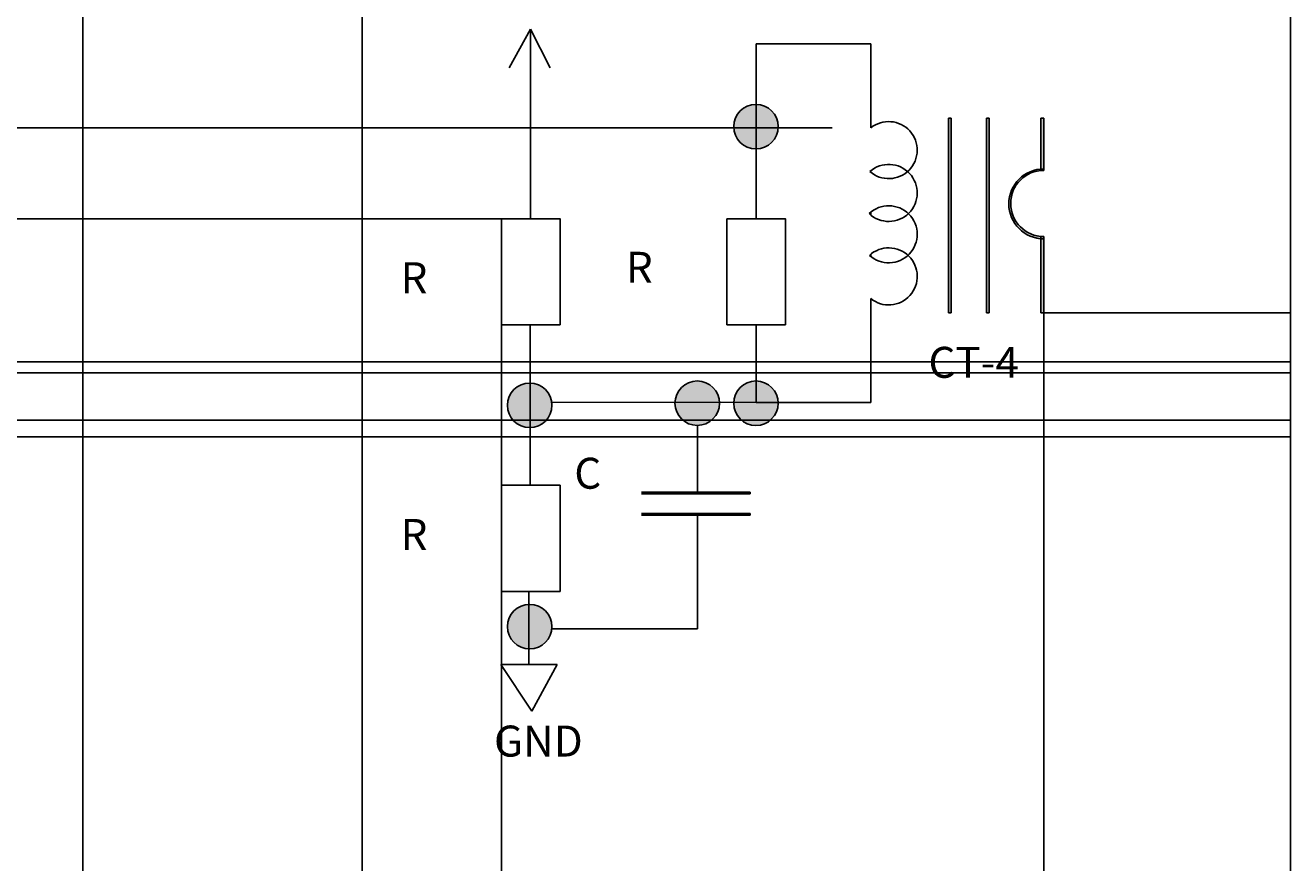
# Model space of a CAD drawing. Units: inches. Extents: x 35362 to 73946, y 43607 to 67532.
# Tile 133 of 134: x 64925 to 73946, y 49781 to 55752. Entities that reach past the tile are written whole.
import ezdxf

# ---------------------------------------------------------------- set-up
doc = ezdxf.new("R2010")
doc.units = ezdxf.units.IN
doc.header["$MEASUREMENT"] = 0
for name, color, linetype, lineweight in [('A-ANNO-DIMS', 2, 'Continuous', 18), ('E-ANNO-TEXT', 5, 'Continuous', 18), ('E-SYMB', 1, 'Continuous', 25), ('E-SYMB-PATT', 1, 'Continuous', 13), ('E-WIRE', 3, 'Continuous', 25)]:
    doc.layers.add(name, color=color, linetype=linetype, lineweight=lineweight)
doc.styles.get("Standard").update_dxf_attribs({"font": 'arial.ttf'})
doc.dimstyles.get("Standard").update_dxf_attribs({"dimtxt": 0.18, "dimasz": 0.18, "dimexe": 0.18, "dimexo": 0.0625, "dimgap": 0.09, "dimtad": 0, "dimtih": 1, "dimtoh": 1, "dimdec": 4, "dimzin": 0, "dimdsep": 46, "dimtxsty": 'Standard', "dimcen": 0.09, "dimadec": 0, "dimazin": 0, "dimtfac": 1, "dimtdec": 4, "dimtofl": 0, "dimtmove": 0, "dimatfit": 3, "dimfxl": 1, "dimtolj": 1, "dimtzin": 0, "dimarcsym": 0})

# ---------------------------------------------------------------- blocks, each defined once
blk = doc.blocks.new('CT-CORE')
for p, q in [((-0.0004610742907971, 1387.996120092102), (-0.0004610742907971, -5.34733626409e-05)), ((19.99953892572375, 1387.996120092102), (-0.0004610742907971, 1387.996120092102)), ((19.9995389257092, -5.34733626409e-05), (19.99953892572375, 1387.996120092102)), ((270.6681283192447, 1387.996120092102), (270.6681283192447, -5.34733626409e-05)), ((290.6681283192593, 1387.996120092102), (270.6681283192447, 1387.996120092102)), ((290.6681283192447, -5.34733626409e-05), (290.6681283192593, 1387.996120092102)), ((658.9826659540267, 1387.996120092102), (658.9826659540267, 1014.585417332389)), ((678.9826659540413, 1387.996120092102), (658.9826659540267, 1387.996120092102)), ((678.9826659540413, 1015.434583844784), (678.9826659540413, 1387.996120092102)), ((658.9826659540267, 544.3844491987692), (658.9826659540267, -5.34733626409e-05)), ((678.9826659540267, -5.34733626409e-05), (678.9826659540413, 543.5352826863744)), ((-0.0004610742907971, -5.34733626409e-05), (19.9995389257092, -5.34733626409e-05)), ((270.6681283192447, -5.34733626409e-05), (290.6681283192447, -5.34733626409e-05)), ((658.9826659540267, -5.34733626409e-05), (678.9826659540267, -5.34733626409e-05))]:
    blk.add_line(p, q)
blk.add_arc((678.9826659540267, 779.4849332655793), 235.9496505792049, 90, 270)
blk = doc.blocks.new('PWR-5V')
for p, q in [((149.83075954589, 1350.920325582869), (-0.0001436721213395, 1075.898385659784)), ((149.83075954589, 833.0941938853575), (149.83075954589, 1350.920325582869)), ((289.9554714129044, 1075.898385659784), (149.83075954589, 1350.920325582869)), ((149.83075954589, 416.3126341884199), (149.83075954589, 833.0941938853575)), ((149.83075954589, 416.3126341884199), (149.83075954589, 0.0003315384019515))]:
    blk.add_line(p, q)
blk = doc.blocks.new('*D6')
at = {"layer": 'A-ANNO-DIMS', "color": 0, "lineweight": -2, "transparency": 16777216}
for p, q in [((72185.645666, 53702.123839), (72185.645666, 43606.678996)), ((69871.496302, 45449.831951), (69871.496302, 43606.678996)), ((69871.67630199999, 43606.858996), (71028.21104539152, 43606.858996)), ((72185.465666, 43606.858996), (71028.93092260844, 43606.858996))]:
    blk.add_line(p, q, dxfattribs=at)
at = {"layer": 'A-ANNO-DIMS', "color": 0, "transparency": 16777216}
for points in [[(69871.67630199999, 43606.888996), (69871.67630199999, 43606.828996), (69871.496302, 43606.858996)], [(72185.465666, 43606.888996), (72185.465666, 43606.828996), (72185.645666, 43606.858996)]]:
    blk.add_solid(points, dxfattribs=at)
at = {"layer": 'Defpoints', "color": 0, "transparency": 16777216}
for p in [(72185.645666, 53702.186339), (69871.496302, 45449.894451), (72185.645666, 43606.858996)]:
    blk.add_point(p, dxfattribs=at)
at = {"layer": 'A-ANNO-DIMS', "color": 0, "transparency": 16777216, "insert": (71028.57098399999, 43606.858996), "char_height": 0.18, "attachment_point": 5}
blk.add_mtext('\\A1;2314', dxfattribs=at)
blk = doc.blocks.new('*D7')
at = {"layer": 'A-ANNO-DIMS', "color": 0, "lineweight": -2, "transparency": 16777216}
for p, q in [((72185.70816600003, 53702.18633900003), (73945.82566600003, 53702.18633900003)), ((73945.64566600005, 53702.00633900003), (73945.64566600005, 49576.22229813781)), ((73945.64566600005, 45450.07445100001), (73945.64566600005, 49575.85849186223)), ((69871.55880200003, 45449.89445100001), (73945.82566600003, 45449.89445100001))]:
    blk.add_line(p, q, dxfattribs=at)
at = {"layer": 'A-ANNO-DIMS', "color": 0, "transparency": 16777216}
for points in [[(73945.61566600006, 53702.00633900003), (73945.67566600005, 53702.00633900003), (73945.64566600005, 53702.18633900003)], [(73945.61566600006, 45450.07445100001), (73945.67566600005, 45450.07445100001), (73945.64566600005, 45449.89445100001)]]:
    blk.add_solid(points, dxfattribs=at)
at = {"layer": 'Defpoints', "color": 0, "transparency": 16777216}
for p in [(72185.64566600003, 53702.18633900003), (73945.64566600005, 53702.18633900003), (69871.49630200001, 45449.89445100001)]:
    blk.add_point(p, dxfattribs=at)
at = {"layer": 'A-ANNO-DIMS', "color": 0, "transparency": 16777216, "insert": (73945.64566600005, 49576.04039499998), "char_height": 0.18, "attachment_point": 5}
blk.add_mtext('\\A1;8252', dxfattribs=at)
blk = doc.blocks.new('*D8')
at = {"layer": 'A-ANNO-DIMS', "color": 0, "lineweight": -2, "transparency": 16777216}
for p, q in [((66271.28651900003, 65771.51172800003), (73945.82566600003, 65771.51172800003)), ((73945.64566600005, 65771.33172800003), (73945.64566600005, 59737.03093663782)), ((73945.64566600005, 53702.36633900002), (73945.64566600005, 59736.66713036224)), ((72185.70816600003, 53702.18633900003), (73945.82566600003, 53702.18633900003))]:
    blk.add_line(p, q, dxfattribs=at)
at = {"layer": 'A-ANNO-DIMS', "color": 0, "transparency": 16777216}
for points in [[(73945.61566600006, 65771.33172800003), (73945.67566600005, 65771.33172800003), (73945.64566600005, 65771.51172800003)], [(73945.61566600006, 53702.36633900002), (73945.67566600005, 53702.36633900002), (73945.64566600005, 53702.18633900003)]]:
    blk.add_solid(points, dxfattribs=at)
at = {"layer": 'Defpoints', "color": 0, "transparency": 16777216}
for p in [(66271.22401900003, 65771.51172800003), (73945.64566600005, 65771.51172800003), (72185.64566600003, 53702.18633900003)]:
    blk.add_point(p, dxfattribs=at)
at = {"layer": 'A-ANNO-DIMS', "color": 0, "transparency": 16777216, "insert": (73945.64566600005, 59736.84903349999), "char_height": 0.18, "attachment_point": 5}
blk.add_mtext('\\A1;12069', dxfattribs=at)
blk = doc.blocks.new('*D10')
at = {"layer": 'A-ANNO-DIMS', "color": 0, "lineweight": -2, "transparency": 16777216}
for p, q in [((61240.96983600002, 59185.14395700003), (73945.82566600003, 59185.14395700003)), ((73945.64566600005, 59184.96395700003), (73945.64566600005, 56268.51827402935)), ((73945.64566600005, 53351.70866200003), (73945.64566600005, 56268.1543449707)), ((61240.96983600002, 53351.52866200003), (73945.82566600003, 53351.52866200003))]:
    blk.add_line(p, q, dxfattribs=at)
at = {"layer": 'A-ANNO-DIMS', "color": 0, "transparency": 16777216}
for points in [[(73945.61566600006, 59184.96395700003), (73945.67566600005, 59184.96395700003), (73945.64566600005, 59185.14395700003)], [(73945.61566600006, 53351.70866200003), (73945.67566600005, 53351.70866200003), (73945.64566600005, 53351.52866200003)]]:
    blk.add_solid(points, dxfattribs=at)
at = {"layer": 'Defpoints', "color": 0, "transparency": 16777216}
for p in [(61240.90733600002, 59185.14395700003), (61240.90733600002, 53351.52866200003), (73945.64566600005, 53351.52866200003)]:
    blk.add_point(p, dxfattribs=at)
at = {"layer": 'A-ANNO-DIMS', "color": 0, "transparency": 16777216, "insert": (73945.64566600005, 56268.33630949999), "char_height": 0.18, "attachment_point": 5}
blk.add_mtext('\\A1;5834', dxfattribs=at)
blk = doc.blocks.new('*D36')
at = {"layer": 'A-ANNO-DIMS', "color": 0, "lineweight": -2, "transparency": 16777216}
for p, q in [((68320.80826200004, 60122.34633200002), (35361.76908500003, 60122.34633200002)), ((35361.94908500003, 60122.16633200002), (35361.94908500003, 57247.82893113781)), ((35361.94908500003, 54373.12772400002), (35361.94908500003, 57247.46512486223)), ((68320.80826200004, 54372.94772400003), (35361.76908500003, 54372.94772400002))]:
    blk.add_line(p, q, dxfattribs=at)
at = {"layer": 'A-ANNO-DIMS', "color": 0, "transparency": 16777216}
for points in [[(35361.91908500003, 60122.16633200002), (35361.97908500003, 60122.16633200002), (35361.94908500003, 60122.34633200002)], [(35361.91908500003, 54373.12772400002), (35361.97908500003, 54373.12772400002), (35361.94908500003, 54372.94772400002)]]:
    blk.add_solid(points, dxfattribs=at)
at = {"layer": 'Defpoints', "color": 0, "transparency": 16777216}
for p in [(68320.87076200004, 60122.34633200002), (35361.94908500003, 54372.94772400002), (68320.87076200004, 54372.94772400003)]:
    blk.add_point(p, dxfattribs=at)
at = {"layer": 'A-ANNO-DIMS', "color": 0, "transparency": 16777216, "insert": (35361.94908500004, 57247.64702799999), "char_height": 0.18, "attachment_point": 5}
blk.add_mtext('\\A1;5749.4', dxfattribs=at)
blk = doc.blocks.new('*D56')
at = {"layer": 'A-ANNO-DIMS', "color": 0, "lineweight": -2, "transparency": 16777216}
for p, q in [((59433.20767900003, 53351.52866200003), (73945.82566600003, 53351.52866200003)), ((73945.64566600005, 53351.34866200002), (73945.64566600005, 53143.55447552935)), ((73945.64566600005, 52935.39636000002), (73945.64566600005, 53143.19054647069)), ((59433.20767900003, 52935.21636000003), (73945.82566600003, 52935.21636000003))]:
    blk.add_line(p, q, dxfattribs=at)
at = {"layer": 'A-ANNO-DIMS', "color": 0, "transparency": 16777216}
for points in [[(73945.61566600006, 53351.34866200002), (73945.67566600005, 53351.34866200002), (73945.64566600005, 53351.52866200003)], [(73945.61566600006, 52935.39636000002), (73945.67566600005, 52935.39636000002), (73945.64566600005, 52935.21636000003)]]:
    blk.add_solid(points, dxfattribs=at)
at = {"layer": 'Defpoints', "color": 0, "transparency": 16777216}
for p in [(59433.14517900002, 53351.52866200003), (59433.14517900002, 52935.21636000003), (73945.64566600005, 52935.21636000003)]:
    blk.add_point(p, dxfattribs=at)
at = {"layer": 'A-ANNO-DIMS', "color": 0, "transparency": 16777216, "insert": (73945.64566600005, 53143.37251099998), "char_height": 0.18, "attachment_point": 5}
blk.add_mtext('\\A1;416.3', dxfattribs=at)
blk = doc.blocks.new('*D57')
at = {"layer": 'A-ANNO-DIMS', "color": 0, "lineweight": -2, "transparency": 16777216}
for p, q in [((51445.41811300003, 53272.78194700003), (73945.82566600003, 53272.78194700003)), ((73945.64566600005, 53272.60194700003), (73945.64566600005, 53045.85764863782)), ((73945.64566600005, 52818.74954400002), (73945.64566600005, 53045.49384236224)), ((51445.41811300003, 52818.56954400002), (73945.82566600003, 52818.56954400002))]:
    blk.add_line(p, q, dxfattribs=at)
at = {"layer": 'A-ANNO-DIMS', "color": 0, "transparency": 16777216}
for points in [[(73945.61566600006, 53272.60194700003), (73945.67566600005, 53272.60194700003), (73945.64566600005, 53272.78194700003)], [(73945.61566600006, 52818.74954400002), (73945.67566600005, 52818.74954400002), (73945.64566600005, 52818.56954400002)]]:
    blk.add_solid(points, dxfattribs=at)
at = {"layer": 'Defpoints', "color": 0, "transparency": 16777216}
for p in [(51445.35561300003, 53272.78194700003), (51445.35561300003, 52818.56954400002), (73945.64566600005, 52818.56954400002)]:
    blk.add_point(p, dxfattribs=at)
at = {"layer": 'A-ANNO-DIMS', "color": 0, "transparency": 16777216, "insert": (73945.64566600005, 53045.6757455), "char_height": 0.18, "attachment_point": 5}
blk.add_mtext('\\A1;454.2', dxfattribs=at)
blk = doc.blocks.new('*D65')
at = {"layer": 'A-ANNO-DIMS', "color": 0, "lineweight": -2, "transparency": 16777216}
for p, q in [((65336.01600799999, 61293.223552), (65336.01600799999, 43606.678996)), ((67326.639741, 61293.223552), (67326.639741, 43606.678996)), ((65336.19600799999, 43606.858996), (66330.87277900206, 43606.858996)), ((67326.45974100001, 43606.858996), (66331.78296999796, 43606.858996))]:
    blk.add_line(p, q, dxfattribs=at)
at = {"layer": 'A-ANNO-DIMS', "color": 0, "transparency": 16777216}
for points in [[(65336.19600799999, 43606.888996), (65336.19600799999, 43606.828996), (65336.01600799999, 43606.858996)], [(67326.45974100001, 43606.888996), (67326.45974100001, 43606.828996), (67326.639741, 43606.858996)]]:
    blk.add_solid(points, dxfattribs=at)
at = {"layer": 'Defpoints', "color": 0, "transparency": 16777216}
for p in [(65336.01600799999, 61293.286052), (67326.639741, 61293.286052), (67326.639741, 43606.858996)]:
    blk.add_point(p, dxfattribs=at)
at = {"layer": 'A-ANNO-DIMS', "color": 0, "transparency": 16777216, "insert": (66331.32787450001, 43606.858996), "char_height": 0.18, "attachment_point": 5}
blk.add_mtext('\\A1;1990.6', dxfattribs=at)
blk = doc.blocks.new('*D68')
at = {"layer": 'A-ANNO-DIMS', "color": 0, "lineweight": -2, "transparency": 16777216}
for p, q in [((68320.870762, 54372.885224), (68320.870762, 43606.678996)), ((61240.907336, 53351.466162), (61240.907336, 43606.678996)), ((61241.08733599999, 43606.858996), (64780.42646373397, 43606.858996)), ((68320.69076200001, 43606.858996), (64781.35163426603, 43606.858996))]:
    blk.add_line(p, q, dxfattribs=at)
at = {"layer": 'A-ANNO-DIMS', "color": 0, "transparency": 16777216}
for points in [[(61241.08733599999, 43606.888996), (61241.08733599999, 43606.828996), (61240.907336, 43606.858996)], [(68320.69076200001, 43606.888996), (68320.69076200001, 43606.828996), (68320.870762, 43606.858996)]]:
    blk.add_solid(points, dxfattribs=at)
at = {"layer": 'Defpoints', "color": 0, "transparency": 16777216}
for p in [(68320.870762, 54372.947724), (61240.907336, 53351.52866199999), (68320.870762, 43606.858996)]:
    blk.add_point(p, dxfattribs=at)
at = {"layer": 'A-ANNO-DIMS', "color": 0, "transparency": 16777216, "insert": (64780.889049, 43606.858996), "char_height": 0.18, "attachment_point": 5}
blk.add_mtext('\\A1;7080.0', dxfattribs=at)

msp = doc.modelspace()

# ---------------------------------------------------------------- hatches: boundary and pattern name
at = {"layer": 'E-SYMB-PATT'}
h = msp.add_hatch(color=256, dxfattribs=at)
h.dxf.hatch_style = 1
h.paths.add_polyline_path([(70135.80528894292, 55188.08141031771, 0.4183931940818975), (69974.93949760578, 55029.49162493918, 0.4183931940818975), (70135.80528894292, 54870.90183956064)])
h.paths.add_polyline_path([(70135.80528894292, 55188.08141031771), (70135.80528894292, 54870.90183956064, 0.4100462469397049), (70292.15127038094, 55029.49162493918, 0.4100462469397049)])
h = msp.add_hatch(color=256, dxfattribs=at)
h.dxf.hatch_style = 1
h.paths.add_polyline_path([(71526.66253892572, 55090.18251302161), (71506.66253892571, 55090.18251302161), (71506.66253892571, 53702.18633945615), (71526.6625389257, 53702.18633945615)])
h = msp.add_hatch(color=256, dxfattribs=at)
h.dxf.hatch_style = 1
h.paths.add_polyline_path([(71797.33112831926, 55090.18251302161), (71777.33112831925, 55090.18251302161), (71777.33112831925, 53702.18633945615), (71797.33112831925, 53702.18633945615)])
h = msp.add_hatch(color=256, dxfattribs=at)
h.dxf.hatch_style = 1
h.paths.add_polyline_path([(72185.64566595404, 54245.72167561588, -0.0212196039209565), (72165.64566595403, 54246.57084212828), (72165.64566595403, 54229.69792765927, 0.0200709024740955), (72185.64566595404, 54228.89476801458)])
h.paths.add_polyline_path([(72185.64566595404, 54228.89476801458, -0.0200709024740953), (72165.64566595403, 54229.69792765927), (72165.64566595403, 53702.18633945615), (72185.64566595403, 53702.18633945615)])
h.paths.add_polyline_path([(72185.64566595404, 55090.18251302161), (72165.64566595403, 55090.18251302161), (72165.64566595403, 54726.92775889016, -0.0200709024740959), (72185.64566595404, 54727.73091853485)])
h.paths.add_polyline_path([(72185.64566595404, 54727.73091853485, 0.020070902474096), (72165.64566595403, 54726.92775889015), (72165.64566595403, 54716.77181026191, -0.0212196039209564), (72185.64566595404, 54717.62097677429)])
h = msp.add_hatch(color=256, dxfattribs=at)
h.dxf.hatch_style = 1
h.paths.add_polyline_path([(72165.64566595403, 54716.77181026191), (72165.64566595403, 54726.92775889016, 0.3908929169039177), (71936.22759069389, 54478.31284327471, 0.3908929169039177), (72165.64566595403, 54229.69792765927), (72165.64566595403, 54246.57084212828, -0.389569854577291), (71949.69601537482, 54481.67132619509, -0.389569854577291)])
h = msp.add_hatch(color=256, dxfattribs=at)
h.dxf.hatch_style = 1
h.paths.add_polyline_path([(68522.99328781641, 53200.70415181951, 0.4183931940818975), (68362.12749647925, 53042.11436644098, 0.4183931940818975), (68522.99328781641, 52883.52458106244)])
h.paths.add_polyline_path([(68522.99328781641, 53200.70415181951), (68522.99328781641, 52883.52458106244, 0.4100462469397049), (68679.33926925441, 53042.11436644098, 0.4100462469397049)])
h = msp.add_hatch(color=256, dxfattribs=at)
h.dxf.hatch_style = 1
h.paths.add_polyline_path([(69717.45127656072, 53215.91996812531, 0.4183931940818975), (69556.58548522356, 53057.33018274678, 0.4183931940818975), (69717.45127656072, 52898.74039736824)])
h.paths.add_polyline_path([(69717.45127656072, 53215.91996812531), (69717.45127656072, 52898.74039736824, 0.4100462469397049), (69873.79725799873, 53057.33018274678, 0.4100462469397049)])
h = msp.add_hatch(color=256, dxfattribs=at)
h.dxf.hatch_style = 1
h.paths.add_polyline_path([(70135.80528894292, 53215.63442430999, 0.4183931940818975), (69974.93949760577, 53057.04463893146, 0.4183931940818975), (70135.80528894292, 52898.45485355292)])
h.paths.add_polyline_path([(70135.80528894292, 53215.63442430999), (70135.80528894292, 52898.45485355292, 0.4100462469397049), (70292.15127038091, 53057.04463893146, 0.4100462469397049)])
h = msp.add_hatch(color=256, dxfattribs=at)
h.dxf.hatch_style = 1
h.paths.add_polyline_path([(70091.40622432147, 52410.91197640568), (70091.40622432147, 52422.06668613867), (69317.27150299007, 52422.06668613867), (69317.27150299007, 52410.91197640569)])
h = msp.add_hatch(color=256, dxfattribs=at)
h.dxf.hatch_style = 1
h.paths.add_polyline_path([(70091.40622432147, 52259.9504989795), (70091.40622432147, 52271.10520871249), (69317.27150299007, 52271.10520871249), (69317.27150299007, 52259.9504989795)])
h = msp.add_hatch(color=256, dxfattribs=at)
h.dxf.hatch_style = 1
h.paths.add_polyline_path([(68522.99328781641, 51622.81584653964, 0.4183931940818975), (68362.12749647925, 51464.2260611611, 0.4183931940818975), (68522.99328781641, 51305.63627578257)])
h.paths.add_polyline_path([(68522.99328781641, 51622.81584653964), (68522.99328781641, 51305.63627578257, 0.4100462469397049), (68679.33926925441, 51464.2260611611, 0.4100462469397049)])

# ---------------------------------------------------------------- linework, layer by layer
at = {"layer": 'E-SYMB'}
for p, q in [((70951.91702453484, 55019.71202248002), (70951.91702453484, 55285.91371364523)), ((70131.22999091068, 55188.0806099024), (70131.22999091068, 55187.39438664135)), ((70135.80528894292, 54875.37298504554), (70135.80528894292, 54870.90183956064)), ((70135.80528894292, 54789.26002711793), (70135.80528894292, 54372.94772446791)), ((70951.91702453484, 54714.44355652491), (70951.91702453484, 54704.26791857422)), ((70951.91702453484, 54419.35072852053), (70951.91702453484, 54398.99945261911)), ((70951.91702453484, 54119.17003350033), (70951.91702453484, 54103.90662461472)), ((70951.91702453484, 53803.72592959452), (70951.91702453484, 53606.10888565044)), ((68522.99328781641, 53346.21373695894), (68522.99328781641, 53616.32943079317)), ((70135.80528894292, 53483.41110146581), (70136.39879188087, 53616.32943079317)), ((70951.91702453484, 53606.10888565044), (70951.91702453484, 53483.41110146581)), ((68518.41798978415, 53200.70335140419), (68518.41798978415, 53200.01712814314)), ((69712.87597852846, 53215.91916771), (69712.87597852846, 53215.23294444895)), ((70131.22999091067, 53215.63362389468), (70131.22999091067, 53214.94740063362)), ((68522.99328781641, 52887.99572654734), (68522.99328781641, 52883.52458106244)), ((69717.45127656072, 52903.21154285314), (69717.45127656072, 52898.74039736824)), ((70135.80528894292, 52902.92599903782), (70135.80528894292, 52898.45485355292)), ((68522.99328781641, 52718.98263901538), (68522.99328781641, 52471.68342389732)), ((69717.45127656072, 52665.14561790383), (69717.45127656074, 52410.91197640568)), ((70091.40622432147, 52422.06668613867), (69317.27150299007, 52422.06668613867)), ((70091.40622432147, 52410.91197640568), (70091.40622432147, 52422.06668613867)), ((69317.27150299007, 52410.91197640569), (70091.40622432147, 52410.91197640568)), ((70091.40622432147, 52271.10520871249), (69317.27150299007, 52271.10520871249)), ((69317.27150299007, 52259.9504989795), (70091.40622432147, 52259.9504989795)), ((69717.45127656074, 52271.10520871249), (69717.45127656072, 51969.55006940491)), ((70091.40622432147, 52259.9504989795), (70091.40622432147, 52271.10520871249)), ((68515.4609857722, 51715.06513022257), (68515.4609857722, 51622.74429047768)), ((68515.4609857722, 51622.74429047768), (68515.4609857722, 51194.1435117944)), ((68518.41798978415, 51622.81504612431), (68518.41798978415, 51622.12882286327)), ((68522.99328781641, 51310.10742126747), (68522.99328781641, 51305.63627578257)), ((68515.4609857722, 51194.1435117944), (68315.4609857722, 51194.1435117944)), ((68315.4609857722, 51194.1435117944), (68537.17167350776, 50861.210529133)), ((68515.4609857722, 51194.1435117944), (68715.4609857722, 51194.1435117944)), ((68537.17167350776, 50861.210529133), (68715.4609857722, 51194.1435117944))]:
    msp.add_line(p, q, dxfattribs=at)
for points in [[(68320.87076221016, 54372.94772446791), (68737.80188109005, 54372.94772446791), (68737.80188109005, 53616.32943079317), (68320.87076221016, 53616.32943079317)], [(69927.32366271509, 54372.94772446791), (70344.25478159498, 54372.94772446791), (70344.25478159498, 53616.32943079317), (69927.32366271509, 53616.32943079317)], [(68320.87076221016, 52471.68342389732), (68737.80188109005, 52471.68342389732), (68737.80188109005, 51715.06513022257), (68320.87076221016, 51715.06513022257)]]:
    msp.add_lwpolyline(points, close=True, dxfattribs=at)
for centre in [(70133.54538399336, 55029.49162493918), (68520.73338286683, 53042.11436644098), (69715.19137161114, 53057.33018274678), (70133.54538399335, 53057.04463893146), (68520.73338286683, 51464.2260611611)]:
    msp.add_circle(centre, 158.6058863875805, dxfattribs=at)
for centre, radius, start, end in [((71080.24668337766, 54861.98997052712), 203.3340773479672, 228.6473573753312, 129.1333314268913), ((71080.24668337766, 54556.72150457201), 203.3340773479672, 226.5217351845822, 131.3526426246687), ((72185.64566595403, 54478.31284327471), 249.4180752601387, 90, 270), ((71080.24668337766, 54261.62867656763), 203.3340773479672, 227.5737684206601, 133.4782648154177), ((71080.24668337766, 53961.44798154742), 203.3340773479672, 230.8666685731087, 132.4262315793399)]:
    msp.add_arc(centre, radius, start, end, dxfattribs=at)
at = {"layer": 'E-WIRE'}
for p, q in [((70135.80528894292, 55206.04158681487), (70135.80528894292, 55620.78745233789)), ((70135.80528894292, 55620.78745233789), (70951.91702453484, 55620.78745233789)), ((70951.91702453484, 55620.78745233789), (70951.91702453484, 55285.91371364523)), ((70135.80528894292, 54789.26002711793), (70135.80528894292, 55206.04158681487)), ((61657.21963859326, 55020.33824525718), (70677.18977032776, 55020.33824525718)), ((70135.80528894292, 53483.41110146581), (70135.80528894292, 53063.39615610514)), ((70951.91702453484, 53063.39615610514), (70951.91702453484, 53483.41110146581)), ((68522.99328781641, 52718.98263901538), (68522.99328781641, 53346.21373695894)), ((70135.80528894292, 53063.39615610514), (68677.76702326702, 53064.39132717303)), ((70135.80528894292, 53063.39615610514), (70951.91702453484, 53063.39615610514)), ((69717.45127656072, 52665.14561790383), (69717.45127656072, 52898.74039736824)), ((69717.45127656069, 51449.09966737698), (69717.45127656072, 51969.55006940491)), ((68678.61631230469, 51449.09966737698), (69717.45127656069, 51449.09966737698))]:
    msp.add_line(p, q, dxfattribs=at)

# ---------------------------------------------------------------- block references
at = {"layer": 'E-SYMB'}
for name, p in [('PWR-5V', (68375.605, 54372.94739292951)), ('CT-CORE', (71506.66299999999, 53702.18639292949))]:
    msp.add_blockref(name, p, dxfattribs=at)

# ---------------------------------------------------------------- texts
at = {"layer": 'E-ANNO-TEXT'}
for s, p in [('R', (69206.76051434176, 53915.85881374982)), ('R', (67600.30761383683, 53841.63876788242)), ('CT-4', (71363.54243146715, 53238.12946447569)), ('C', (68838.78053002528, 52447.37656697481)), ('R', (67600.30761383683, 52010.96463123842)), ('GND', (68266.33050224229, 50537.38209495451))]:
    msp.add_text(s, height=220.8659825270206, dxfattribs=at).set_placement(p)

# ---------------------------------------------------------------- dimensions: what is measured, and where the dimension line sits
at = {"layer": 'A-ANNO-DIMS'}
for base, p1, p2, override, picture, middle in [((73945.64566600005, 65771.51172800003), (72185.645666, 53702.186339), (66271.224019, 65771.51172799998), {"dimdec": 0, "dimlfac": 1, "dimrnd": 0, "dimzin": 0, "dimdsep": 46, "dimlunit": 2}, '*D8', (73945.64566600005, 59736.84903349999)), ((35361.94908500003, 54372.94772400002), (68320.870762, 60122.346332), (68320.870762, 54372.947724), {"dimdec": 1, "dimlfac": 1, "dimrnd": 0, "dimzin": 0, "dimdsep": 46, "dimlunit": 2}, '*D36', (35361.94908500004, 57247.64702799999)), ((73945.64566600005, 53351.52866200003), (61240.907336, 59185.14395699999), (61240.907336, 53351.52866199999), {"dimdec": 0, "dimlfac": 1, "dimrnd": 0, "dimzin": 0, "dimdsep": 46, "dimlunit": 2}, '*D10', (73945.64566600005, 56268.33630949999)), ((73945.64566600005, 53702.18633900003), (69871.496302, 45449.894451), (72185.645666, 53702.186339), {"dimdec": 0, "dimlfac": 1, "dimrnd": 0, "dimzin": 0, "dimdsep": 46, "dimlunit": 2}, '*D7', (73945.64566600005, 49576.04039499998)), ((73945.64566600005, 52935.21636000003), (59433.145179, 53351.52866199999), (59433.145179, 52935.21636), {"dimdec": 1, "dimlfac": 1, "dimrnd": 0, "dimzin": 0, "dimdsep": 46, "dimlunit": 2}, '*D56', (73945.64566600005, 53143.37251099998)), ((73945.64566600005, 52818.56954400002), (51445.355613, 53272.781947), (51445.355613, 52818.569544), {"dimdec": 1, "dimlfac": 1, "dimrnd": 0, "dimzin": 0, "dimdsep": 46, "dimlunit": 2}, '*D57', (73945.64566600005, 53045.6757455))]:
    dim = msp.add_linear_dim(base=base, p1=p1, p2=p2, angle=90, dimstyle='Standard', override=override, dxfattribs=at)
    dim.commit()
    dim.dimension.update_dxf_attribs({"geometry": picture, "text_midpoint": middle})
for base, p1, p2, override, picture, middle in [((67326.639741, 43606.858996), (65336.01600799999, 61293.286052), (67326.639741, 61293.286052), {"dimdec": 1, "dimlfac": 1, "dimrnd": 0, "dimzin": 0, "dimdsep": 46, "dimlunit": 2}, '*D65', (66331.32787450001, 43606.858996)), ((68320.870762, 43606.858996), (61240.907336, 53351.52866199999), (68320.870762, 54372.947724), {"dimdec": 1, "dimlfac": 1, "dimrnd": 0, "dimzin": 0, "dimdsep": 46, "dimlunit": 2}, '*D68', (64780.889049, 43606.858996)), ((72185.645666, 43606.858996), (69871.496302, 45449.894451), (72185.645666, 53702.186339), {"dimdec": 0, "dimlfac": 1, "dimrnd": 0, "dimzin": 0, "dimdsep": 46, "dimlunit": 2}, '*D6', (71028.57098399999, 43606.858996))]:
    dim = msp.add_linear_dim(base=base, p1=p1, p2=p2, dimstyle='Standard', override=override, dxfattribs=at)
    dim.commit()
    dim.dimension.update_dxf_attribs({"geometry": picture, "text_midpoint": middle})

doc.saveas('drawing.dxf')
